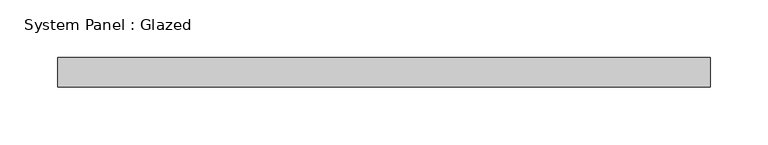
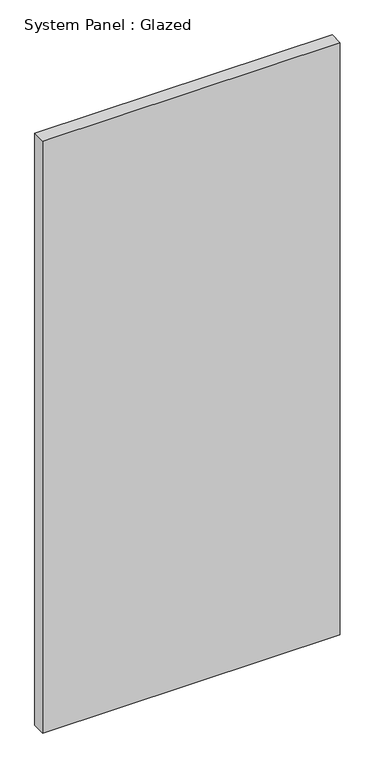
"""IFC4 building model written with IfcOpenShell, lengths in millimetres: plate geometry, System Panel : Glazed."""

from ifc_helpers import new_model, si_unit, origin, origin_with_axes, place, context, project, spatial, polyline, outline, extrude, source, transform, mapped, element, save


def system_panel_glazed_65e788ca(model_context):
    return source(origin(), model_context, "Body", "SweptSolid", [
        extrude(outline(polyline([(282.575, 19.05), (-282.575, 19.05), (-282.575, 44.45), (282.575, 44.45), (282.575, 19.05)])), origin_with_axes(), (0.0, 0.0, 1.0), 1188.425758),
    ])


if __name__ == "__main__":
    model = new_model("IFC4")
    model_context = context("Model", 3, world=origin())
    ifc_project = project(units=[si_unit("LENGTHUNIT", "METRE", prefix="MILLI")], contexts=[model_context])
    site = spatial("IfcSite", under=ifc_project)
    building = spatial("IfcBuilding", under=site)
    placement = place(None, origin())
    system_panel_glazed_shape = system_panel_glazed_65e788ca(model_context)
    element("IfcPlate", 1, ObjectType="System Panel : Glazed", at=placement, inside=building, context=model_context, shape_type="MappedRepresentation", body=[
        mapped(system_panel_glazed_shape, transform((0.0, 0.0, 0.0), x_axis=(1.0, 0.0, 0.0), y_axis=(0.0, 1.0, 0.0), z_axis=(0.0, 0.0, 1.0))),
    ])
    save(model, "model.ifc")

# Revit data of these elements
# Type "System Panel : Glazed"
#   Construction Type Id = "GSP4R"
#   Analytic Construction = "1/8 in Pilkington single glazing"
#   Visual Light Transmittance = 0.9
#   Solar Heat Gain Coefficient = 0.86
#   Heat Transfer Coefficient (U) = 1.18115 BTU/(h·ft²·°F)
#   Define Thermal Properties by = 1
# Element 1 (IfcPlate, "System Panel : Glazed")
#   Materials on its faces: "Glass"
# Materials
#   "Glass": class "Glass", colour RGB 0 128 192, transparency 0.75, Description = "Soda Lime Glass", Cost = 0
